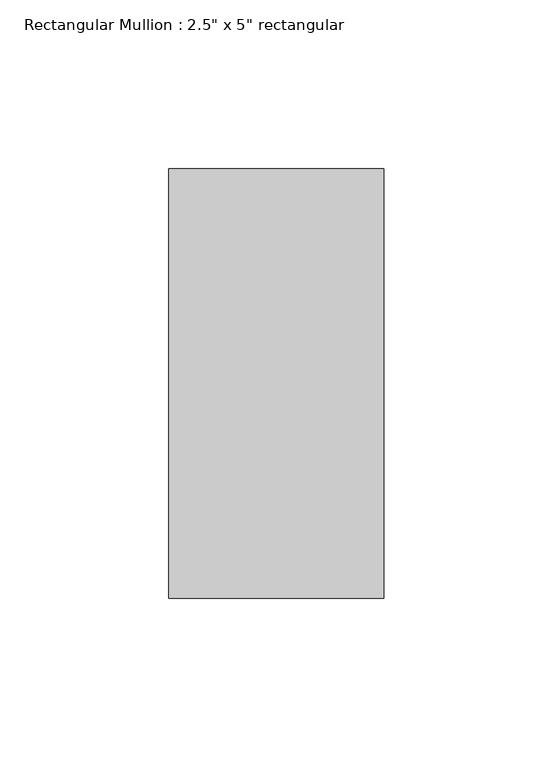
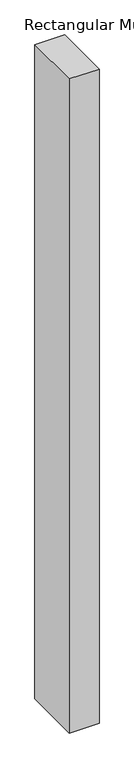
"""IFC4 building model written with IfcOpenShell, lengths in millimetres: member geometry."""

from ifc_helpers import new_model, si_unit, frame, origin, place, context, project, spatial, polyline, outline, extrude, source, transform, mapped, element, save


def member_852981e0(model_context):
    return source(origin(), model_context, "Body", "SweptSolid", [
        extrude(outline(polyline([(0.0, 63.5), (0.0, -63.5), (-63.5, -63.5), (-63.5, 63.5), (0.0, 63.5)])), frame((0.0, 0.0, -1475.7821201), z_axis=(0.0, 0.0, 1.0), x_axis=(1.0, 0.0, 0.0)), (0.0, 0.0, 1.0), 1475.7821201),
    ])


if __name__ == "__main__":
    model = new_model("IFC4")
    model_context = context("Model", 3, world=origin())
    ifc_project = project(units=[si_unit("LENGTHUNIT", "METRE", prefix="MILLI")], contexts=[model_context])
    site = spatial("IfcSite", under=ifc_project)
    building = spatial("IfcBuilding", under=site)
    placement = place(None, origin())
    member_shape = member_852981e0(model_context)
    element("IfcMember", 1, ObjectType="Rectangular Mullion : 2.5\" x 5\" rectangular", at=placement, inside=building, context=model_context, shape_type="MappedRepresentation", body=[
        mapped(member_shape, transform((0.0, 0.0, 0.0), x_axis=(1.0, 0.0, 0.0), y_axis=(0.0, 1.0, 0.0), z_axis=(0.0, 0.0, 1.0))),
    ])
    save(model, "model.ifc")

# Revit data of these elements
# Type "Rectangular Mullion : 2.5\" x 5\" rectangular"
#   built-in parameter 1007304 = 0.416667 (stored number, unit not read)
#   built-in parameter 1007301 = 0.104167 (stored number, unit not read)
#   built-in parameter 1007300 = 0.104167 (stored number, unit not read)
# Element 1 (IfcMember, "Rectangular Mullion : 2.5\" x 5\" rectangular")
#   Materials on its faces: "Aluminum"
# Materials
#   "Aluminum": class "Metal", colour RGB 247 247 247, transparency 0, Description = "Aluminum 6061", Cost = 0
